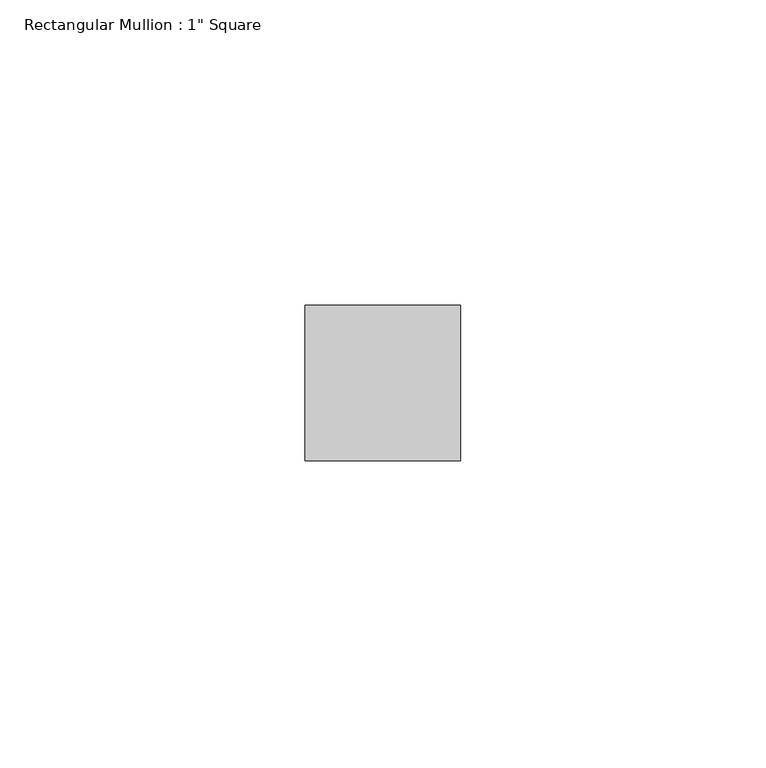
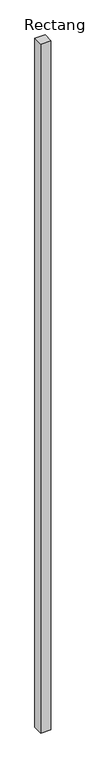
"""IFC4 building model written with IfcOpenShell, lengths in millimetres: member geometry."""

from ifc_helpers import new_model, si_unit, frame, origin, place, context, project, spatial, polyline, outline, extrude, source, transform, mapped, element, save


def member_1744d714(model_context):
    return source(origin(), model_context, "Body", "SweptSolid", [
        extrude(outline(polyline([(12.7, 12.7), (12.7, -12.7), (-12.7, -12.7), (-12.7, 12.7), (12.7, 12.7)])), frame((0.0, 0.0, -1828.8), z_axis=(0.0, 0.0, 1.0), x_axis=(1.0, 0.0, 0.0)), (0.0, 0.0, 1.0), 1828.8),
    ])


if __name__ == "__main__":
    model = new_model("IFC4")
    model_context = context("Model", 3, world=origin())
    ifc_project = project(units=[si_unit("LENGTHUNIT", "METRE", prefix="MILLI")], contexts=[model_context])
    site = spatial("IfcSite", under=ifc_project)
    building = spatial("IfcBuilding", under=site)
    placement = place(None, origin())
    member_shape = member_1744d714(model_context)
    element("IfcMember", 1, ObjectType="Rectangular Mullion : 1\" Square", at=placement, inside=building, context=model_context, shape_type="MappedRepresentation", body=[
        mapped(member_shape, transform((0.0, 0.0, 0.0), x_axis=(1.0, 0.0, 0.0), y_axis=(0.0, 1.0, 0.0), z_axis=(0.0, 0.0, 1.0))),
    ])
    save(model, "model.ifc")

# Revit data of these elements
# Type "Rectangular Mullion : 1\" Square"
#   built-in parameter 1007304 = 0.0833333 (stored number, unit not read)
#   built-in parameter 1007301 = 0.0416667 (stored number, unit not read)
#   built-in parameter 1007300 = 0.0416667 (stored number, unit not read)
# Element 1 (IfcMember, "Rectangular Mullion : 1\" Square")
#   Materials on its faces: "Aluminum"
# Materials
#   "Aluminum": class "Metal", colour RGB 247 247 247, transparency 0, Description = "Aluminum 6061", Cost = 0
